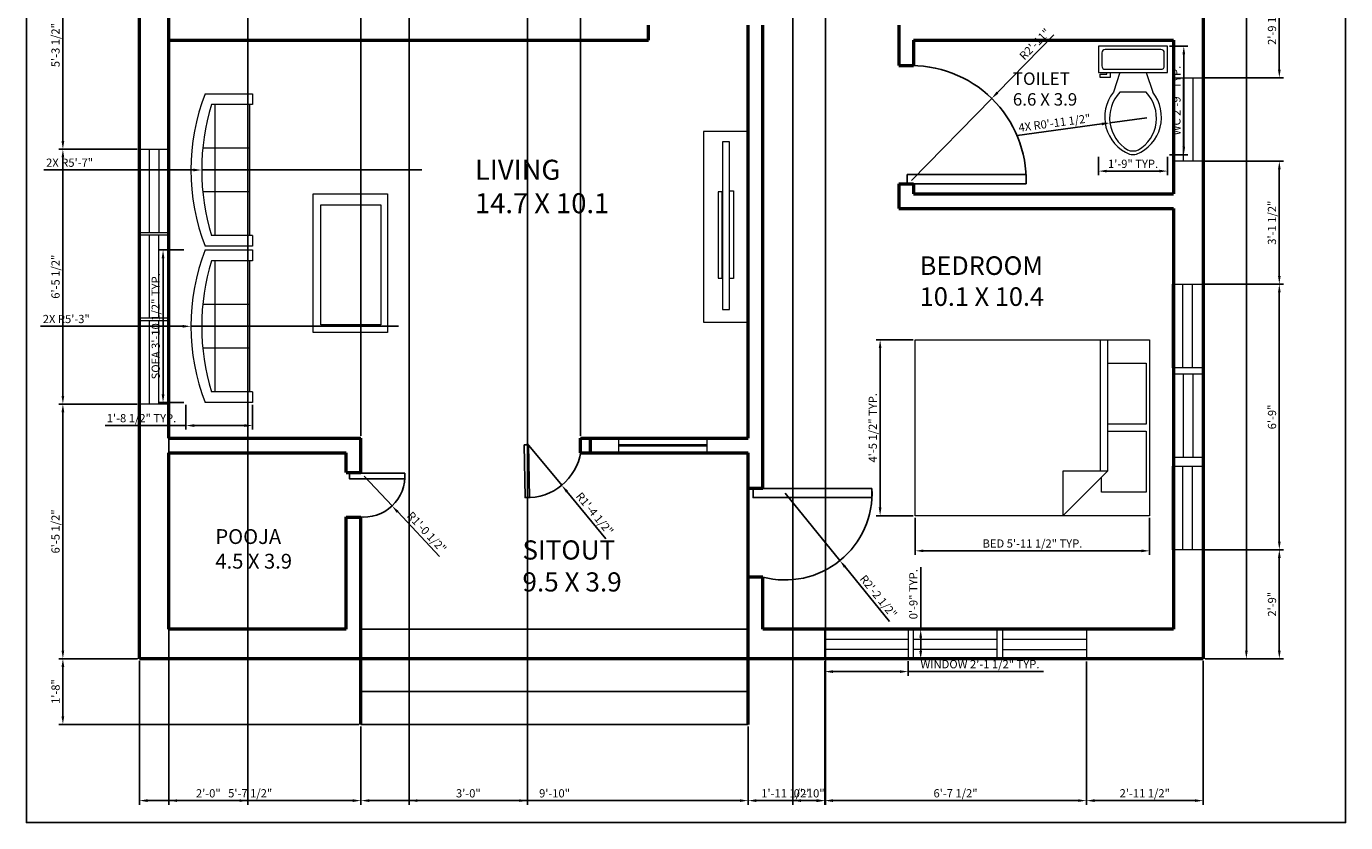
# Model space of a CAD drawing. Units: inches. Extents: x 231 to 633, y -1 to 510.
# Tile 1 of 3: x 231 to 633, y -1 to 242. Entities that reach past the tile are written whole.
import ezdxf

# ---------------------------------------------------------------- set-up
doc = ezdxf.new("R2010")
doc.units = ezdxf.units.IN
for name, color, linetype, lineweight in [('A-ANNO-DIMS', 2, 'Continuous', 18), ('A-ANNO-TTLB', 7, 'Continuous', 25), ('A-AREA-IDEN', 7, 'Continuous', 25), ('A-DOOR', 3, 'Continuous', 25), ('A-FLOR-FIXT', 9, 'Continuous', 18), ('A-FLOR-STRS', 7, 'Continuous', 25), ('A-FURN', 8, 'Continuous', 18), ('A-GLAZ', 4, 'Continuous', 18), ('A-WALL', 7, 'Continuous', 50)]:
    doc.layers.add(name, color=color, linetype=linetype, lineweight=lineweight)
doc.styles.get("Standard").update_dxf_attribs({"font": 'arial.ttf'})
doc.dimstyles.new('ISO-25', dxfattribs={"dimtxt": 2.5, "dimasz": 2.5, "dimexe": 1.25, "dimexo": 0.625, "dimtad": 1, "dimtxsty": 'Standard', "dimcen": 2.5, "dimadec": 0, "dimazin": 0, "dimtfac": 1, "dimtmove": 0, "dimatfit": 3, "dimfxl": 1, "dimarcsym": 0})

# ---------------------------------------------------------------- blocks, each defined once
blk = doc.blocks.new('Sofa - Roundback 7 ft.')
for p, q in [((-12.00002, -32.4421), (-12.00003, -6.5971)), ((11.99997, -32.4421), (11.99998, -6.5971)), ((-36.000027, -34), (-36.000027, -11.4696)), ((-35.999844, -13.3819), (35.9998, -13.3819)), ((35.99998, -34), (35.99998, -11.4696)), ((-36.000027, -32.4421), (35.99998, -32.4421))]:
    blk.add_line(p, q)
for points in [[(-36.000027, -34), (-42.000027, -34), (-42.000027, -8)], [(41.99998, -8), (41.99998, -34), (35.99998, -34)]]:
    blk.add_lwpolyline(points)
for centre, radius, start, end in [((0, -114.25), 114.25, 68.43141, 111.5686), ((-0.00001, -127.1968), 121.1968, 72.72033, 107.2797)]:
    blk.add_arc(centre, radius, start, end)
blk = doc.blocks.new('Toilet - top')
for p, q in [((9.5, -6), (9.5, -2)), ((-8, -8.5), (-8, -8)), ((-7, -8), (-7, -9.5)), ((-4, -8), (-6, -14)), ((4, -8), (6, -14)), ((-10, -8.5), (-8, -8.5)), ((-10, -9.5), (-10, -8.5)), ((-7, -9.5), (-10, -9.5)), ((4, -14), (-4, -14))]:
    blk.add_line(p, q)
blk.add_lwpolyline([(10.5, -8), (10.5, 0), (-10.5, 0), (-10.5, -8)], close=True)
for points in [[(-9.5, -2), (-9.5, -6)], [(8.5, -1), (-8.5, -1)], [(-8.5, -7), (8.5, -7)]]:
    blk.add_lwpolyline(points)
for centre, radius, start, end in [((-8.62, -1.88), 0.884, 81.8699, 188.1301), ((8.62, -1.88), 0.884, 351.8699, 98.1301), ((-8.62, -6.12), 0.884, 171.8699, 278.1301), ((8.62, -6.12), 0.884, 261.8699, 8.1301), ((3.52, -21.58), 12.17, 141.4691, 247.9714), ((4.2, -21.82), 11.33, 136.3677, 238.9468), ((-3.52, -21.58), 12.17, 292.0284, 38.5307), ((-4.2, -21.82), 11.33, 301.053, 43.6321), ((0, -27.88), 4, 245.7318, 294.2682), ((0, -29), 4, 254.8605, 285.1395)]:
    blk.add_arc(centre, radius, start, end)
blk = doc.blocks.new('Bed - Queen')
for p, q in [((0, -80.00003), (0, 0)), ((0, 0), (59.99999, 0)), ((59.99999, 0), (59.99999, -80.00003)), ((7.99999, -1.2), (28.79998, -1.2)), ((7.99999, -14.4), (7.99999, -1.2)), ((28.79998, -1.2), (28.79998, -14.4)), ((31.19999, -1.2), (51.99999, -1.2)), ((31.19999, -14.4), (31.19999, -1.2)), ((51.99999, -1.2), (51.99999, -16.4)), ((0, -14.4), (44.8, -14.4)), ((44.8, -16.8), (0, -16.8)), ((59.99999, -29.6), (44.8, -14.4)), ((44.8, -14.4), (44.8, -29.6)), ((51.99999, -16.4), (46.79936, -16.4)), ((44.8, -29.6), (59.99999, -29.6)), ((59.99999, -80.00003), (0, -80.00003))]:
    blk.add_line(p, q)
blk = doc.blocks.new('*D9')
at = {"layer": 'A-ANNO-DIMS', "color": 0, "lineweight": -2, "transparency": 16777216}
for p, q in [((589.91, 469.03), (603.7, 469.03)), ((602.45, 466.53), (602.45, 51.53)), ((589.91, 49.03), (603.7, 49.03))]:
    blk.add_line(p, q, dxfattribs=at)
at = {"layer": 'A-ANNO-DIMS', "color": 0, "transparency": 16777216}
for points in [[(602.04, 466.53), (602.87, 466.53), (602.45, 469.03)], [(602.04, 51.53), (602.87, 51.53), (602.45, 49.03)]]:
    blk.add_solid(points, dxfattribs=at)
at = {"layer": 'Defpoints', "color": 0, "transparency": 16777216}
for p in [(589.28, 469.03), (589.28, 49.03), (602.45, 49.03)]:
    blk.add_point(p, dxfattribs=at)
at = {"layer": 'A-ANNO-DIMS', "color": 0, "transparency": 16777216, "insert": (601.32, 259.03), "char_height": 1, "attachment_point": 5, "rotation": 90}
blk.add_mtext("35'", dxfattribs=at)
blk = doc.blocks.new('WIN-25_43x9')
for p, q in [((0, 0), (0, 9)), ((0, 9), (25.43, 9)), ((25.43, 9), (25.43, 0)), ((25.43, 6), (0, 6)), ((0, 3), (25.43, 3)), ((25.43, 0), (0, 0))]:
    blk.add_line(p, q)
blk = doc.blocks.new('*D12')
at = {"layer": 'A-ANNO-DIMS', "color": 0, "lineweight": -2, "transparency": 16777216}
for p, q in [((474.01, 48.31), (474.01, 43.87)), ((499.44, 48.31), (499.44, 43.87)), ((476.51, 45.12), (496.94, 45.12)), ((499.44, 45.12), (540.65, 45.12))]:
    blk.add_line(p, q, dxfattribs=at)
at = {"layer": 'A-ANNO-DIMS', "color": 0, "transparency": 16777216}
for points in [[(476.51, 45.53), (476.51, 44.7), (474.01, 45.12)], [(496.94, 45.53), (496.94, 44.7), (499.44, 45.12)]]:
    blk.add_solid(points, dxfattribs=at)
at = {"layer": 'Defpoints', "color": 0, "transparency": 16777216}
for p in [(474.01, 48.93), (499.44, 48.93), (499.44, 45.12)]:
    blk.add_point(p, dxfattribs=at)
at = {"layer": 'A-ANNO-DIMS', "color": 0, "transparency": 16777216, "insert": (521.3, 47.04), "char_height": 2.5, "attachment_point": 5}
blk.add_mtext('WINDOW 2\'-1 1/2" TYP.', dxfattribs=at)
blk = doc.blocks.new('*D13')
at = {"layer": 'A-ANNO-DIMS', "color": 0, "lineweight": -2, "transparency": 16777216}
for p, q in [((503.26, 57.93), (503.26, 76.92)), ((500.07, 57.93), (504.51, 57.93)), ((503.26, 51.43), (503.26, 55.43)), ((500.07, 48.93), (504.51, 48.93))]:
    blk.add_line(p, q, dxfattribs=at)
at = {"layer": 'A-ANNO-DIMS', "color": 0, "transparency": 16777216}
for points in [[(502.84, 55.43), (503.67, 55.43), (503.26, 57.93)], [(502.84, 51.43), (503.67, 51.43), (503.26, 48.93)]]:
    blk.add_solid(points, dxfattribs=at)
at = {"layer": 'Defpoints', "color": 0, "transparency": 16777216}
for p in [(499.44, 57.93), (503.26, 57.93), (499.44, 48.93)]:
    blk.add_point(p, dxfattribs=at)
at = {"layer": 'A-ANNO-DIMS', "color": 0, "transparency": 16777216, "insert": (501.35, 68.68), "char_height": 2.5, "attachment_point": 5, "rotation": 90}
blk.add_mtext('0\'-9" TYP.', dxfattribs=at)
blk = doc.blocks.new('*D14')
at = {"layer": 'A-ANNO-DIMS', "color": 0, "lineweight": -2, "transparency": 16777216}
for p, q in [((501.6, 91.97), (501.6, 80.64)), ((572.99, 91.97), (572.99, 80.64)), ((504.1, 81.89), (570.49, 81.89))]:
    blk.add_line(p, q, dxfattribs=at)
at = {"layer": 'A-ANNO-DIMS', "color": 0, "transparency": 16777216}
for points in [[(504.1, 82.3), (504.1, 81.47), (501.6, 81.89)], [(570.49, 82.3), (570.49, 81.47), (572.99, 81.89)]]:
    blk.add_solid(points, dxfattribs=at)
at = {"layer": 'Defpoints', "color": 0, "transparency": 16777216}
for p in [(501.6, 92.59), (572.99, 92.59), (572.99, 81.89)]:
    blk.add_point(p, dxfattribs=at)
at = {"layer": 'A-ANNO-DIMS', "color": 0, "transparency": 16777216, "insert": (537.3, 83.8), "char_height": 2.5, "attachment_point": 5}
blk.add_mtext('BED 5\'-11 1/2" TYP.', dxfattribs=at)
blk = doc.blocks.new('*D15')
at = {"layer": 'A-ANNO-DIMS', "color": 0, "lineweight": -2, "transparency": 16777216}
for p, q in [((500.98, 146.13), (489.65, 146.13)), ((490.9, 143.63), (490.9, 95.09)), ((500.98, 92.59), (489.65, 92.59))]:
    blk.add_line(p, q, dxfattribs=at)
at = {"layer": 'A-ANNO-DIMS', "color": 0, "transparency": 16777216}
for points in [[(490.48, 143.63), (491.31, 143.63), (490.9, 146.13)], [(490.48, 95.09), (491.31, 95.09), (490.9, 92.59)]]:
    blk.add_solid(points, dxfattribs=at)
at = {"layer": 'Defpoints', "color": 0, "transparency": 16777216}
for p in [(501.6, 146.13), (490.9, 92.59), (501.6, 92.59)]:
    blk.add_point(p, dxfattribs=at)
at = {"layer": 'A-ANNO-DIMS', "color": 0, "transparency": 16777216, "insert": (488.98, 119.36), "char_height": 2.5, "attachment_point": 5, "rotation": 90}
blk.add_mtext('4\'-5 1/2" TYP.', dxfattribs=at)
blk = doc.blocks.new('*D16')
at = {"layer": 'A-ANNO-DIMS', "color": 0, "lineweight": -2, "transparency": 16777216}
for p, q in [((579.07, 235.52), (584.65, 235.52)), ((583.4, 204.97), (583.4, 233.02)), ((579.07, 202.47), (584.65, 202.47))]:
    blk.add_line(p, q, dxfattribs=at)
at = {"layer": 'A-ANNO-DIMS', "color": 0, "transparency": 16777216}
for points in [[(582.98, 233.02), (583.82, 233.02), (583.4, 235.52)], [(582.98, 204.97), (583.82, 204.97), (583.4, 202.47)]]:
    blk.add_solid(points, dxfattribs=at)
at = {"layer": 'Defpoints', "color": 0, "transparency": 16777216}
for p in [(578.44, 235.52), (583.4, 235.52), (578.44, 202.47)]:
    blk.add_point(p, dxfattribs=at)
at = {"layer": 'A-ANNO-DIMS', "color": 0, "transparency": 16777216, "insert": (581.48, 218.99), "char_height": 2.5, "attachment_point": 5, "rotation": 90}
blk.add_mtext('WC 2\'-9" TYP.', dxfattribs=at)
blk = doc.blocks.new('*D17')
at = {"layer": 'A-ANNO-DIMS', "color": 0, "lineweight": -2, "transparency": 16777216}
for p, q in [((557.44, 201.85), (557.44, 196.26)), ((578.44, 201.85), (578.44, 196.26)), ((559.94, 197.51), (575.94, 197.51))]:
    blk.add_line(p, q, dxfattribs=at)
at = {"layer": 'A-ANNO-DIMS', "color": 0, "transparency": 16777216}
for points in [[(559.94, 197.93), (559.94, 197.1), (557.44, 197.51)], [(575.94, 197.93), (575.94, 197.1), (578.44, 197.51)]]:
    blk.add_solid(points, dxfattribs=at)
at = {"layer": 'Defpoints', "color": 0, "transparency": 16777216}
for p in [(557.44, 202.47), (578.44, 202.47), (578.44, 197.51)]:
    blk.add_point(p, dxfattribs=at)
at = {"layer": 'A-ANNO-DIMS', "color": 0, "transparency": 16777216, "insert": (567.94, 199.41), "char_height": 2.5, "attachment_point": 5}
blk.add_mtext('1\'-9" TYP.', dxfattribs=at)
blk = doc.blocks.new('*D18')
at = {"layer": 'A-ANNO-DIMS', "color": 0, "lineweight": -2, "transparency": 16777216}
for p, q in [((278.84, 173.5), (271.24, 173.5)), ((272.49, 129.51), (272.49, 171)), ((278.84, 127.01), (271.24, 127.01))]:
    blk.add_line(p, q, dxfattribs=at)
at = {"layer": 'A-ANNO-DIMS', "color": 0, "transparency": 16777216}
for points in [[(272.08, 171), (272.91, 171), (272.49, 173.5)], [(272.08, 129.51), (272.91, 129.51), (272.49, 127.01)]]:
    blk.add_solid(points, dxfattribs=at)
at = {"layer": 'Defpoints', "color": 0, "transparency": 16777216}
for p in [(272.49, 173.5), (279.47, 173.5), (279.47, 127.01)]:
    blk.add_point(p, dxfattribs=at)
at = {"layer": 'A-ANNO-DIMS', "color": 0, "transparency": 16777216, "insert": (270.58, 150.26), "char_height": 2.5, "attachment_point": 5, "rotation": 90}
blk.add_mtext('SOFA 3\'-10 1/2" TYP.', dxfattribs=at)
blk = doc.blocks.new('*D19')
at = {"layer": 'A-ANNO-DIMS', "color": 0, "lineweight": -2, "transparency": 16777216}
for p, q in [((279.47, 126.39), (279.47, 118.79)), ((299.76, 126.39), (299.76, 118.79)), ((279.47, 120.04), (254.89, 120.04)), ((297.26, 120.04), (281.97, 120.04))]:
    blk.add_line(p, q, dxfattribs=at)
at = {"layer": 'A-ANNO-DIMS', "color": 0, "transparency": 16777216}
for points in [[(281.97, 120.46), (281.97, 119.62), (279.47, 120.04)], [(297.26, 120.46), (297.26, 119.62), (299.76, 120.04)]]:
    blk.add_solid(points, dxfattribs=at)
at = {"layer": 'Defpoints', "color": 0, "transparency": 16777216}
for p in [(279.47, 127.01), (299.76, 127.01), (279.47, 120.04)]:
    blk.add_point(p, dxfattribs=at)
at = {"layer": 'A-ANNO-DIMS', "color": 0, "transparency": 16777216, "insert": (265.93, 121.96), "char_height": 2.5, "attachment_point": 5}
blk.add_mtext('1\'-8 1/2" TYP.', dxfattribs=at)
blk = doc.blocks.new('*D30')
at = {"layer": 'A-ANNO-DIMS', "color": 0, "lineweight": -2, "transparency": 16777216}
for p, q in [((264.66, 49.03), (240.73, 49.03)), ((241.98, 31.53), (241.98, 46.53)), ((332.16, 29.03), (240.73, 29.03))]:
    blk.add_line(p, q, dxfattribs=at)
at = {"layer": 'A-ANNO-DIMS', "color": 0, "transparency": 16777216}
for points in [[(241.56, 46.53), (242.4, 46.53), (241.98, 49.03)], [(241.56, 31.53), (242.4, 31.53), (241.98, 29.03)]]:
    blk.add_solid(points, dxfattribs=at)
at = {"layer": 'Defpoints', "color": 0, "transparency": 16777216}
for p in [(241.98, 49.03), (265.28, 49.03), (332.78, 29.03)]:
    blk.add_point(p, dxfattribs=at)
at = {"layer": 'A-ANNO-DIMS', "color": 0, "transparency": 16777216, "insert": (240.08, 39.03), "char_height": 2.5, "attachment_point": 5, "rotation": 90}
blk.add_mtext('1\'-8"', dxfattribs=at)
blk = doc.blocks.new('*D31')
at = {"layer": 'A-ANNO-DIMS', "color": 0, "lineweight": -2, "transparency": 16777216}
for p, q in [((265.28, 48.41), (265.28, 4.58)), ((332.78, 28.41), (332.78, 4.58)), ((267.78, 5.83), (330.28, 5.83))]:
    blk.add_line(p, q, dxfattribs=at)
at = {"layer": 'A-ANNO-DIMS', "color": 0, "transparency": 16777216}
for points in [[(267.78, 6.25), (267.78, 5.42), (265.28, 5.83)], [(330.28, 6.25), (330.28, 5.42), (332.78, 5.83)]]:
    blk.add_solid(points, dxfattribs=at)
at = {"layer": 'Defpoints', "color": 0, "transparency": 16777216}
for p in [(265.28, 49.03), (332.78, 29.03), (332.78, 5.83)]:
    blk.add_point(p, dxfattribs=at)
at = {"layer": 'A-ANNO-DIMS', "color": 0, "transparency": 16777216, "insert": (299.03, 7.75), "char_height": 2.5, "attachment_point": 5}
blk.add_mtext('5\'-7 1/2"', dxfattribs=at)
blk = doc.blocks.new('*D32')
at = {"layer": 'A-ANNO-DIMS', "color": 0, "lineweight": -2, "transparency": 16777216}
for p, q in [((332.78, 28.41), (332.78, 4.58)), ((450.68, 28.41), (450.68, 4.58)), ((335.28, 5.83), (448.18, 5.83))]:
    blk.add_line(p, q, dxfattribs=at)
at = {"layer": 'A-ANNO-DIMS', "color": 0, "transparency": 16777216}
for points in [[(335.28, 6.25), (335.28, 5.42), (332.78, 5.83)], [(448.18, 6.25), (448.18, 5.42), (450.68, 5.83)]]:
    blk.add_solid(points, dxfattribs=at)
at = {"layer": 'Defpoints', "color": 0, "transparency": 16777216}
for p in [(332.78, 29.03), (450.68, 29.03), (450.68, 5.83)]:
    blk.add_point(p, dxfattribs=at)
at = {"layer": 'A-ANNO-DIMS', "color": 0, "transparency": 16777216, "insert": (391.73, 7.73), "char_height": 2.5, "attachment_point": 5}
blk.add_mtext('9\'-10"', dxfattribs=at)
blk = doc.blocks.new('*D35')
at = {"layer": 'A-ANNO-DIMS', "color": 0, "lineweight": -2, "transparency": 16777216}
for p, q in [((464.28, 330.11), (464.28, 4.58)), ((474.28, 330.11), (474.28, 4.58)), ((466.78, 5.83), (471.78, 5.83))]:
    blk.add_line(p, q, dxfattribs=at)
at = {"layer": 'A-ANNO-DIMS', "color": 0, "transparency": 16777216}
for points in [[(466.78, 6.25), (466.78, 5.42), (464.28, 5.83)], [(471.78, 6.25), (471.78, 5.42), (474.28, 5.83)]]:
    blk.add_solid(points, dxfattribs=at)
at = {"layer": 'Defpoints', "color": 0, "transparency": 16777216}
for p in [(464.28, 330.73), (474.28, 330.73), (474.28, 5.83)]:
    blk.add_point(p, dxfattribs=at)
at = {"layer": 'A-ANNO-DIMS', "color": 0, "transparency": 16777216, "insert": (469.28, 7.73), "char_height": 2.5, "attachment_point": 5}
blk.add_mtext('0\'-10"', dxfattribs=at)
blk = doc.blocks.new('*D41')
at = {"layer": 'A-ANNO-DIMS', "color": 0, "lineweight": -2, "transparency": 16777216}
for p, q in [((274.28, 349.01), (274.28, 4.58)), ((298.28, 349.01), (298.28, 4.58)), ((276.78, 5.83), (295.78, 5.83))]:
    blk.add_line(p, q, dxfattribs=at)
at = {"layer": 'A-ANNO-DIMS', "color": 0, "transparency": 16777216}
for points in [[(276.78, 6.25), (276.78, 5.42), (274.28, 5.83)], [(295.78, 6.25), (295.78, 5.42), (298.28, 5.83)]]:
    blk.add_solid(points, dxfattribs=at)
at = {"layer": 'Defpoints', "color": 0, "transparency": 16777216}
for p in [(274.28, 349.63), (298.28, 349.63), (298.28, 5.83)]:
    blk.add_point(p, dxfattribs=at)
at = {"layer": 'A-ANNO-DIMS', "color": 0, "transparency": 16777216, "insert": (286.28, 7.73), "char_height": 2.5, "attachment_point": 5}
blk.add_mtext('2\'-0"', dxfattribs=at)
blk = doc.blocks.new('*D42')
at = {"layer": 'A-ANNO-DIMS', "color": 0, "lineweight": -2, "transparency": 16777216}
for p, q in [((347.48, 344.51), (347.48, 4.58)), ((383.48, 330.11), (383.48, 4.58)), ((349.98, 5.83), (380.98, 5.83))]:
    blk.add_line(p, q, dxfattribs=at)
at = {"layer": 'A-ANNO-DIMS', "color": 0, "transparency": 16777216}
for points in [[(349.98, 6.25), (349.98, 5.42), (347.48, 5.83)], [(380.98, 6.25), (380.98, 5.42), (383.48, 5.83)]]:
    blk.add_solid(points, dxfattribs=at)
at = {"layer": 'Defpoints', "color": 0, "transparency": 16777216}
for p in [(347.48, 345.13), (383.48, 330.73), (383.48, 5.83)]:
    blk.add_point(p, dxfattribs=at)
at = {"layer": 'A-ANNO-DIMS', "color": 0, "transparency": 16777216, "insert": (365.48, 7.73), "char_height": 2.5, "attachment_point": 5}
blk.add_mtext('3\'-0"', dxfattribs=at)
blk = doc.blocks.new('*D43')
at = {"layer": 'A-ANNO-DIMS', "color": 0, "lineweight": -2, "transparency": 16777216}
for p, q in [((264.62, 126.57), (240.73, 126.57)), ((241.98, 51.53), (241.98, 124.07)), ((264.66, 49.03), (240.73, 49.03))]:
    blk.add_line(p, q, dxfattribs=at)
at = {"layer": 'A-ANNO-DIMS', "color": 0, "transparency": 16777216}
for points in [[(241.56, 124.07), (242.4, 124.07), (241.98, 126.57)], [(241.56, 51.53), (242.4, 51.53), (241.98, 49.03)]]:
    blk.add_solid(points, dxfattribs=at)
at = {"layer": 'Defpoints', "color": 0, "transparency": 16777216}
for p in [(241.98, 126.57), (265.25, 126.57), (265.28, 49.03)]:
    blk.add_point(p, dxfattribs=at)
at = {"layer": 'A-ANNO-DIMS', "color": 0, "transparency": 16777216, "insert": (240.06, 87.8), "char_height": 2.5, "attachment_point": 5, "rotation": 90}
blk.add_mtext('6\'-5 1/2"', dxfattribs=at)
blk = doc.blocks.new('*D44')
at = {"layer": 'A-ANNO-DIMS', "color": 0, "lineweight": -2, "transparency": 16777216}
for p, q in [((264.65, 204.16), (240.73, 204.16)), ((241.98, 129.07), (241.98, 201.66)), ((264.62, 126.57), (240.73, 126.57))]:
    blk.add_line(p, q, dxfattribs=at)
at = {"layer": 'A-ANNO-DIMS', "color": 0, "transparency": 16777216}
for points in [[(241.56, 201.66), (242.4, 201.66), (241.98, 204.16)], [(241.56, 129.07), (242.4, 129.07), (241.98, 126.57)]]:
    blk.add_solid(points, dxfattribs=at)
at = {"layer": 'Defpoints', "color": 0, "transparency": 16777216}
for p in [(241.98, 204.16), (265.27, 204.16), (265.25, 126.57)]:
    blk.add_point(p, dxfattribs=at)
at = {"layer": 'A-ANNO-DIMS', "color": 0, "transparency": 16777216, "insert": (240.06, 165.36), "char_height": 2.5, "attachment_point": 5, "rotation": 90}
blk.add_mtext('6\'-5 1/2"', dxfattribs=at)
blk = doc.blocks.new('*D45')
at = {"layer": 'A-ANNO-DIMS', "color": 0, "lineweight": -2, "transparency": 16777216}
for p, q in [((264.59, 267.58), (240.73, 267.58)), ((241.98, 206.66), (241.98, 265.08)), ((264.65, 204.16), (240.73, 204.16))]:
    blk.add_line(p, q, dxfattribs=at)
at = {"layer": 'A-ANNO-DIMS', "color": 0, "transparency": 16777216}
for points in [[(241.56, 265.08), (242.4, 265.08), (241.98, 267.58)], [(241.56, 206.66), (242.4, 206.66), (241.98, 204.16)]]:
    blk.add_solid(points, dxfattribs=at)
at = {"layer": 'Defpoints', "color": 0, "transparency": 16777216}
for p in [(241.98, 267.58), (265.22, 267.58), (265.27, 204.16)]:
    blk.add_point(p, dxfattribs=at)
at = {"layer": 'A-ANNO-DIMS', "color": 0, "transparency": 16777216, "insert": (240.06, 235.87), "char_height": 2.5, "attachment_point": 5, "rotation": 90}
blk.add_mtext('5\'-3 1/2"', dxfattribs=at)
blk = doc.blocks.new('*D50')
at = {"layer": 'A-ANNO-DIMS', "color": 0, "lineweight": -2, "transparency": 16777216}
for p, q in [((589.63, 82.23), (613.74, 82.23)), ((612.49, 51.53), (612.49, 79.73)), ((589.91, 49.03), (613.74, 49.03))]:
    blk.add_line(p, q, dxfattribs=at)
at = {"layer": 'A-ANNO-DIMS', "color": 0, "transparency": 16777216}
for points in [[(612.08, 79.73), (612.91, 79.73), (612.49, 82.23)], [(612.08, 51.53), (612.91, 51.53), (612.49, 49.03)]]:
    blk.add_solid(points, dxfattribs=at)
at = {"layer": 'Defpoints', "color": 0, "transparency": 16777216}
for p in [(589, 82.23), (612.49, 82.23), (589.28, 49.03)]:
    blk.add_point(p, dxfattribs=at)
at = {"layer": 'A-ANNO-DIMS', "color": 0, "transparency": 16777216, "insert": (610.59, 65.63), "char_height": 2.5, "attachment_point": 5, "rotation": 90}
blk.add_mtext('2\'-9"', dxfattribs=at)
blk = doc.blocks.new('*D51')
at = {"layer": 'A-ANNO-DIMS', "color": 0, "lineweight": -2, "transparency": 16777216}
for p, q in [((589.63, 163.09), (613.74, 163.09)), ((612.49, 84.73), (612.49, 160.59)), ((589.63, 82.23), (613.74, 82.23))]:
    blk.add_line(p, q, dxfattribs=at)
at = {"layer": 'A-ANNO-DIMS', "color": 0, "transparency": 16777216}
for points in [[(612.08, 160.59), (612.91, 160.59), (612.49, 163.09)], [(612.08, 84.73), (612.91, 84.73), (612.49, 82.23)]]:
    blk.add_solid(points, dxfattribs=at)
at = {"layer": 'Defpoints', "color": 0, "transparency": 16777216}
for p in [(589, 163.09), (612.49, 163.09), (589, 82.23)]:
    blk.add_point(p, dxfattribs=at)
at = {"layer": 'A-ANNO-DIMS', "color": 0, "transparency": 16777216, "insert": (610.59, 122.66), "char_height": 2.5, "attachment_point": 5, "rotation": 90}
blk.add_mtext('6\'-9"', dxfattribs=at)
blk = doc.blocks.new('*D52')
at = {"layer": 'A-ANNO-DIMS', "color": 0, "lineweight": -2, "transparency": 16777216}
for p, q in [((589.84, 200.51), (613.74, 200.51)), ((612.49, 165.59), (612.49, 198.01)), ((589.63, 163.09), (613.74, 163.09))]:
    blk.add_line(p, q, dxfattribs=at)
at = {"layer": 'A-ANNO-DIMS', "color": 0, "transparency": 16777216}
for points in [[(612.08, 198.01), (612.91, 198.01), (612.49, 200.51)], [(612.08, 165.59), (612.91, 165.59), (612.49, 163.09)]]:
    blk.add_solid(points, dxfattribs=at)
at = {"layer": 'Defpoints', "color": 0, "transparency": 16777216}
for p in [(589.22, 200.51), (612.49, 200.51), (589, 163.09)]:
    blk.add_point(p, dxfattribs=at)
at = {"layer": 'A-ANNO-DIMS', "color": 0, "transparency": 16777216, "insert": (610.57, 181.8), "char_height": 2.5, "attachment_point": 5, "rotation": 90}
blk.add_mtext('3\'-1 1/2"', dxfattribs=at)
blk = doc.blocks.new('*D53')
at = {"layer": 'A-ANNO-DIMS', "color": 0, "lineweight": -2, "transparency": 16777216}
for p, q in [((589.78, 259.34), (613.74, 259.34)), ((612.49, 228.44), (612.49, 256.84)), ((589.84, 225.94), (613.74, 225.94))]:
    blk.add_line(p, q, dxfattribs=at)
at = {"layer": 'A-ANNO-DIMS', "color": 0, "transparency": 16777216}
for points in [[(612.08, 256.84), (612.91, 256.84), (612.49, 259.34)], [(612.08, 228.44), (612.91, 228.44), (612.49, 225.94)]]:
    blk.add_solid(points, dxfattribs=at)
at = {"layer": 'Defpoints', "color": 0, "transparency": 16777216}
for p in [(589.15, 259.34), (612.49, 259.34), (589.22, 225.94)]:
    blk.add_point(p, dxfattribs=at)
at = {"layer": 'A-ANNO-DIMS', "color": 0, "transparency": 16777216, "insert": (610.58, 242.64), "char_height": 2.5, "attachment_point": 5, "rotation": 90}
blk.add_mtext('2\'-9 1/2"', dxfattribs=at)
blk = doc.blocks.new('*D61')
at = {"layer": 'A-ANNO-DIMS', "color": 0, "lineweight": -2, "transparency": 16777216}
for p, q in [((474.01, 48.31), (474.01, 4.58)), ((450.68, 28.41), (450.68, 4.58)), ((453.18, 5.83), (471.51, 5.83))]:
    blk.add_line(p, q, dxfattribs=at)
at = {"layer": 'A-ANNO-DIMS', "color": 0, "transparency": 16777216}
for points in [[(453.18, 6.25), (453.18, 5.42), (450.68, 5.83)], [(471.51, 6.25), (471.51, 5.42), (474.01, 5.83)]]:
    blk.add_solid(points, dxfattribs=at)
at = {"layer": 'Defpoints', "color": 0, "transparency": 16777216}
for p in [(474.01, 48.93), (450.68, 29.03), (474.01, 5.83)]:
    blk.add_point(p, dxfattribs=at)
at = {"layer": 'A-ANNO-DIMS', "color": 0, "transparency": 16777216, "insert": (462.35, 7.75), "char_height": 2.5, "attachment_point": 5}
blk.add_mtext('1\'-11 1/2"', dxfattribs=at)
blk = doc.blocks.new('*D62')
at = {"layer": 'A-ANNO-DIMS', "color": 0, "lineweight": -2, "transparency": 16777216}
for p, q in [((553.73, 48.23), (553.73, 4.58)), ((589.28, 48.41), (589.28, 4.58)), ((556.23, 5.83), (586.78, 5.83))]:
    blk.add_line(p, q, dxfattribs=at)
at = {"layer": 'A-ANNO-DIMS', "color": 0, "transparency": 16777216}
for points in [[(556.23, 6.25), (556.23, 5.42), (553.73, 5.83)], [(586.78, 6.25), (586.78, 5.42), (589.28, 5.83)]]:
    blk.add_solid(points, dxfattribs=at)
at = {"layer": 'Defpoints', "color": 0, "transparency": 16777216}
for p in [(553.73, 48.85), (589.28, 49.03), (589.28, 5.83)]:
    blk.add_point(p, dxfattribs=at)
at = {"layer": 'A-ANNO-DIMS', "color": 0, "transparency": 16777216, "insert": (571.5, 7.75), "char_height": 2.5, "attachment_point": 5}
blk.add_mtext('2\'-11 1/2"', dxfattribs=at)
blk = doc.blocks.new('*D63')
at = {"layer": 'A-ANNO-DIMS', "color": 0, "lineweight": -2, "transparency": 16777216}
for p, q in [((474.01, 48.31), (474.01, 4.58)), ((553.73, 48.23), (553.73, 4.58)), ((476.51, 5.83), (551.23, 5.83))]:
    blk.add_line(p, q, dxfattribs=at)
at = {"layer": 'A-ANNO-DIMS', "color": 0, "transparency": 16777216}
for points in [[(476.51, 6.25), (476.51, 5.42), (474.01, 5.83)], [(551.23, 6.25), (551.23, 5.42), (553.73, 5.83)]]:
    blk.add_solid(points, dxfattribs=at)
at = {"layer": 'Defpoints', "color": 0, "transparency": 16777216}
for p in [(474.01, 48.93), (553.73, 48.85), (553.73, 5.83)]:
    blk.add_point(p, dxfattribs=at)
at = {"layer": 'A-ANNO-DIMS', "color": 0, "transparency": 16777216, "insert": (513.87, 7.75), "char_height": 2.5, "attachment_point": 5}
blk.add_mtext('6\'-7 1/2"', dxfattribs=at)
blk = doc.blocks.new('*D65')
at = {"layer": 'A-ANNO-DIMS', "color": 0, "lineweight": -2, "transparency": 16777216}
for p, q in [((332.78, 116.86), (332.78, 493.62)), ((335.28, 492.37), (397.18, 492.37)), ((399.68, 116.86), (399.68, 493.62))]:
    blk.add_line(p, q, dxfattribs=at)
at = {"layer": 'A-ANNO-DIMS', "color": 0, "transparency": 16777216}
for points in [[(335.28, 492.78), (335.28, 491.95), (332.78, 492.37)], [(397.18, 492.78), (397.18, 491.95), (399.68, 492.37)]]:
    blk.add_solid(points, dxfattribs=at)
at = {"layer": 'Defpoints', "color": 0, "transparency": 16777216}
for p in [(399.68, 492.37), (332.78, 116.23), (399.68, 116.23)]:
    blk.add_point(p, dxfattribs=at)
at = {"layer": 'A-ANNO-DIMS', "color": 0, "transparency": 16777216, "insert": (366.23, 494.26), "char_height": 2.5, "attachment_point": 5}
blk.add_mtext('5\'-7"', dxfattribs=at)
blk = doc.blocks.new('*D66')
at = {"layer": 'A-ANNO-DIMS', "color": 0, "lineweight": -2, "transparency": 16777216}
for p, q in [((543.86, 238.98), (526.64, 221.42)), ((500.42, 194.67), (524.89, 219.64))]:
    blk.add_line(p, q, dxfattribs=at)
at = {"layer": 'A-ANNO-DIMS', "color": 0, "transparency": 16777216}
blk.add_solid([(526.35, 221.71), (526.94, 221.13), (524.89, 219.64)], dxfattribs=at)
at = {"layer": 'Defpoints', "color": 0, "transparency": 16777216}
for p in [(524.89, 219.64), (500.42, 194.67)]:
    blk.add_point(p, dxfattribs=at)
at = {"layer": 'A-ANNO-DIMS', "color": 0, "transparency": 16777216, "insert": (538.24, 235.93), "char_height": 2.5, "attachment_point": 5, "rotation": 45.5699}
blk.add_mtext('R2\'-11"', dxfattribs=at)
blk = doc.blocks.new('*D69')
at = {"layer": 'A-ANNO-DIMS', "color": 0, "lineweight": -2, "transparency": 16777216}
for p, q in [((461.99, 99.49), (478.65, 78.93)), ((493.72, 60.33), (480.22, 76.99))]:
    blk.add_line(p, q, dxfattribs=at)
at = {"layer": 'A-ANNO-DIMS', "color": 0, "transparency": 16777216}
blk.add_solid([(480.55, 77.25), (479.9, 76.72), (478.65, 78.93)], dxfattribs=at)
at = {"layer": 'Defpoints', "color": 0, "transparency": 16777216}
for p in [(461.99, 99.49), (478.65, 78.93)]:
    blk.add_point(p, dxfattribs=at)
at = {"layer": 'A-ANNO-DIMS', "color": 0, "transparency": 16777216, "insert": (490.14, 67.8), "char_height": 2.5, "attachment_point": 5, "rotation": 309.0212}
blk.add_mtext('R2\'-2 1/2"', dxfattribs=at)
blk = doc.blocks.new('*D70')
at = {"layer": 'A-ANNO-DIMS', "color": 0, "lineweight": -2, "transparency": 16777216}
for p, q in [((383.44, 114.59), (393.92, 101.86)), ((407.34, 85.56), (395.51, 99.93))]:
    blk.add_line(p, q, dxfattribs=at)
at = {"layer": 'A-ANNO-DIMS', "color": 0, "transparency": 16777216}
blk.add_solid([(395.83, 100.19), (395.19, 99.66), (393.92, 101.86)], dxfattribs=at)
at = {"layer": 'Defpoints', "color": 0, "transparency": 16777216}
for p in [(383.44, 114.59), (393.92, 101.86)]:
    blk.add_point(p, dxfattribs=at)
at = {"layer": 'A-ANNO-DIMS', "color": 0, "transparency": 16777216, "insert": (403.7, 93), "char_height": 2.5, "attachment_point": 5, "rotation": 309.4659}
blk.add_mtext('R1\'-4 1/2"', dxfattribs=at)
blk = doc.blocks.new('*D71')
at = {"layer": 'A-ANNO-DIMS', "color": 0, "lineweight": -2, "transparency": 16777216}
for p, q in [((333.74, 104.6), (342.24, 95.55)), ((356.7, 80.17), (343.96, 93.73))]:
    blk.add_line(p, q, dxfattribs=at)
at = {"layer": 'A-ANNO-DIMS', "color": 0, "transparency": 16777216}
blk.add_solid([(344.26, 94.02), (343.65, 93.45), (342.24, 95.55)], dxfattribs=at)
at = {"layer": 'Defpoints', "color": 0, "transparency": 16777216}
for p in [(333.74, 104.6), (342.24, 95.55)]:
    blk.add_point(p, dxfattribs=at)
at = {"layer": 'A-ANNO-DIMS', "color": 0, "transparency": 16777216, "insert": (352.58, 87.35), "char_height": 2.5, "attachment_point": 5, "rotation": 313.2146}
blk.add_mtext('R1\'-0 1/2"', dxfattribs=at)
blk = doc.blocks.new('*D72')
at = {"layer": 'A-ANNO-DIMS', "color": 0, "lineweight": -2, "transparency": 16777216}
for p, q in [((236.17, 197.85), (281.76, 197.85)), ((351.33, 197.85), (284.26, 197.85))]:
    blk.add_line(p, q, dxfattribs=at)
at = {"layer": 'A-ANNO-DIMS', "color": 0, "transparency": 16777216}
blk.add_solid([(281.76, 198.27), (281.76, 197.44), (284.26, 197.85)], dxfattribs=at)
at = {"layer": 'Defpoints', "color": 0, "transparency": 16777216}
for p in [(284.26, 197.85), (351.33, 197.85)]:
    blk.add_point(p, dxfattribs=at)
at = {"layer": 'A-ANNO-DIMS', "color": 0, "transparency": 16777216, "insert": (244.02, 199.75), "char_height": 2.5, "attachment_point": 5, "rotation": 0.0001}
blk.add_mtext('2X R5\'-7"', dxfattribs=at)
blk = doc.blocks.new('*D73')
at = {"layer": 'A-ANNO-DIMS', "color": 0, "lineweight": -2, "transparency": 16777216}
for p, q in [((235.16, 150.26), (278.44, 150.26)), ((344.17, 150.26), (280.94, 150.26))]:
    blk.add_line(p, q, dxfattribs=at)
at = {"layer": 'A-ANNO-DIMS', "color": 0, "transparency": 16777216}
blk.add_solid([(278.44, 150.67), (278.44, 149.84), (280.94, 150.26)], dxfattribs=at)
at = {"layer": 'Defpoints', "color": 0, "transparency": 16777216}
for p in [(280.94, 150.26), (344.17, 150.26)]:
    blk.add_point(p, dxfattribs=at)
at = {"layer": 'A-ANNO-DIMS', "color": 0, "transparency": 16777216, "insert": (243.01, 152.16), "char_height": 2.5, "attachment_point": 5}
blk.add_mtext('2X R5\'-3"', dxfattribs=at)
blk = doc.blocks.new('*D75')
at = {"layer": 'A-ANNO-DIMS', "color": 0, "lineweight": -2, "transparency": 16777216}
for p, q in [((572.14, 213.7), (560.91, 212.19)), ((532.64, 208.39), (558.44, 211.86))]:
    blk.add_line(p, q, dxfattribs=at)
at = {"layer": 'A-ANNO-DIMS', "color": 0, "transparency": 16777216}
blk.add_solid([(558.38, 212.27), (558.49, 211.44), (560.91, 212.19)], dxfattribs=at)
at = {"layer": 'Defpoints', "color": 0, "transparency": 16777216}
for p in [(572.14, 213.7), (560.91, 212.19)]:
    blk.add_point(p, dxfattribs=at)
at = {"layer": 'A-ANNO-DIMS', "color": 0, "transparency": 16777216, "insert": (544.04, 211.86), "char_height": 2.5, "attachment_point": 5, "rotation": 7.6557}
blk.add_mtext('4X R0\'-11 1/2"', dxfattribs=at)

msp = doc.modelspace()

# ---------------------------------------------------------------- linework, layer by layer
at = {"layer": 'A-ANNO-TTLB'}
msp.add_lwpolyline([(230.86, 510.42), (632.68, 510.42), (632.68, -0.86), (230.86, -0.86)], close=True, dxfattribs=at)
at = {"layer": 'A-DOOR'}
for points in [[(535.37, 196.43), (535.37, 193.68), (499.17, 193.68), (499.17, 196.43)], [(384.11, 98.11), (382.76, 98.11), (382.51, 114.14), (383.85, 114.14)], [(346.13, 105.52), (346.13, 103.85), (329.27, 103.85), (329.27, 105.52)], [(488.42, 100.86), (488.42, 98.12), (452.21, 98.12), (452.21, 100.86)]]:
    msp.add_lwpolyline(points, close=True, dxfattribs=at)
for centre, radius, start, end in [((500.42, 194.67), 34.96, 358.3635, 92.7769), ((383.44, 114.59), 16.49, 267.6488, 351.2829), ((333.74, 104.6), 12.42, 262.1598, 4.268), ((461.99, 99.49), 26.47, 255.0643, 2.9785)]:
    msp.add_arc(centre, radius, start, end, dxfattribs=at)
at = {"layer": 'A-FLOR-STRS'}
for p, q in [((450.68, 58.03), (332.78, 58.03)), ((450.68, 39.03), (332.78, 39.03)), ((450.68, 29.03), (332.78, 29.03))]:
    msp.add_line(p, q, dxfattribs=at)
at = {"layer": 'A-FURN'}
for points in [[(450.56, 209.54), (437.09, 209.54), (437.09, 151.48), (450.56, 151.48)], [(445.02, 206.42), (442.84, 206.42), (442.84, 155.37), (445.02, 155.37)], [(318.24, 190.64), (340.82, 190.64), (340.82, 148.34), (318.24, 148.34)], [(442.83, 191.24), (441.57, 191.24), (441.57, 164.88), (442.83, 164.88)], [(445.04, 191.54), (446.27, 191.54), (446.27, 164.83), (445.04, 164.83)], [(320.54, 187.27), (338.83, 187.27), (338.83, 150.71), (320.54, 150.71)]]:
    msp.add_lwpolyline(points, close=True, dxfattribs=at)
at = {"layer": 'A-GLAZ'}
for p, q in [((411.28, 111.74), (411.28, 116.24)), ((411.28, 116.24), (438.14, 116.24)), ((411.28, 114.24), (438.14, 114.24)), ((438.14, 113.74), (411.28, 113.74)), ((438.14, 116.24), (438.14, 111.74)), ((438.14, 111.74), (411.28, 111.74))]:
    msp.add_line(p, q, dxfattribs=at)
at = {"layer": 'A-WALL'}
for p, q in [((265.28, 49.03), (265.28, 469.03)), ((589.28, 469.03), (589.28, 49.03)), ((274.28, 116.23), (274.28, 345.13)), ((420.38, 237.43), (420.38, 241.93)), ((450.68, 116.23), (450.68, 241.93)), ((455.18, 100.93), (455.18, 241.93)), ((496.58, 241.93), (496.58, 229.63)), ((274.28, 237.43), (420.38, 237.43)), ((501.08, 237.43), (580.28, 237.43)), ((501.08, 237.43), (501.08, 229.63)), ((580.28, 237.43), (580.28, 190.63)), ((496.58, 229.63), (501.08, 229.63)), ((496.58, 193.63), (501.08, 193.63)), ((496.58, 193.63), (496.58, 186.13)), ((501.08, 193.63), (501.08, 190.63)), ((501.08, 190.63), (580.28, 190.63)), ((496.58, 186.13), (580.28, 186.13)), ((580.28, 186.13), (580.28, 58.03)), ((274.28, 116.23), (332.78, 116.23)), ((332.78, 105.73), (332.78, 116.23)), ((399.68, 116.23), (450.68, 116.23)), ((399.68, 111.73), (399.68, 116.23)), ((402.68, 111.73), (402.68, 116.23)), ((274.28, 58.03), (274.28, 111.73)), ((274.28, 111.73), (328.28, 111.73)), ((328.28, 105.73), (328.28, 111.73)), ((399.68, 111.73), (450.68, 111.73)), ((450.68, 100.93), (450.68, 111.73)), ((328.28, 105.73), (332.78, 105.73)), ((450.68, 29.03), (450.68, 100.93)), ((450.68, 100.93), (455.18, 100.93)), ((328.28, 58.03), (328.28, 92.26)), ((328.28, 92.17), (332.78, 92.17)), ((332.78, 29.03), (332.78, 92.22)), ((450.68, 73.93), (455.18, 73.93)), ((455.18, 58.03), (455.18, 73.93)), ((328.28, 58.03), (274.28, 58.03)), ((580.28, 58.03), (455.18, 58.03)), ((589.28, 49.03), (265.28, 49.03))]:
    msp.add_line(p, q, dxfattribs=at)

# ---------------------------------------------------------------- block references
at = {"layer": 'A-FLOR-FIXT'}
msp.add_blockref('Toilet - top', (567.94, 235.52), dxfattribs=at)
at = {"layer": 'A-FURN'}
for name, p, xscale, yscale, zscale, rotation in [('Sofa - Roundback 7 ft.', (280.94, 197.85), 0.5533813357364022, 0.5533813357364022, 0.5533813357364022, 90), ('Sofa - Roundback 7 ft.', (280.94, 150.26), 0.5533813357364022, 0.5533813357364022, 0.5533813357364022, 90), ('Bed - Queen', (572.99, 146.13), 0.8923370876530633, 0.8923370876530633, 0.8923370876530633, 270)]:
    msp.add_blockref(name, p, dxfattribs=dict(at, xscale=xscale, yscale=yscale, zscale=zscale, rotation=rotation))
at = {"layer": 'A-GLAZ'}
for p, rotation in [((580.22, 225.94), 269.9999999999996), ((265.27, 204.16), 270.0000000000001), ((265.25, 178.15), 270), ((580, 163.09), 269.9999999999997), ((265.25, 152), 269.9999999999998), ((580.21, 135.78), 270.0000000000001), ((580, 107.66), 269.9999999999996)]:
    msp.add_blockref('WIN-25_43x9', p, dxfattribs=dict(at, rotation=rotation))
for p in [(474.01, 48.93), (501.03, 48.93), (528.3, 48.85)]:
    msp.add_blockref('WIN-25_43x9', p, dxfattribs=at)

# ---------------------------------------------------------------- texts
at = {"layer": 'A-AREA-IDEN', "attachment_point": 1}
for s, width, gutter_width, insert, char_height in [('TOILET\\P6.6 X 3.9', 27.8521, 18.92, (531.33, 227.55), 3.785), ('LIVING\\P14.7 X 10.1', 110.5251, 30.53, (367.51, 200.97), 6.1055), ('BEDROOM\\P10.1 X 10.4', 154.4931, 28.28, (502.96, 171.56), 5.6558), ('POOJA\\P4.5 X 3.9', 49.8485, 22.53, (288.43, 88.49), 4.506), ('SITOUT\\P9.5 X 3.9', 116.2795, 29.18, (381.95, 85.07), 5.836)]:
    msp.add_mtext_dynamic_manual_height_columns(s, width=width, gutter_width=gutter_width, heights=[0], dxfattribs=dict(at, insert=insert, char_height=char_height))

# ---------------------------------------------------------------- dimensions: what is measured, and where the dimension line sits
at = {"layer": 'A-ANNO-DIMS'}
for base, p1, p2, picture, middle in [((399.68, 492.37), (332.78, 116.23), (399.68, 116.23), '*D65', (366.23, 494.26)), ((298.28, 5.83), (274.28, 349.63), (298.28, 349.63), '*D41', (286.28, 7.73)), ((383.48, 5.83), (347.48, 345.13), (383.48, 330.73), '*D42', (365.48, 7.73)), ((474.28, 5.83), (464.28, 330.73), (474.28, 330.73), '*D35', (469.28, 7.73)), ((332.78, 5.83), (265.28, 49.03), (332.78, 29.03), '*D31', (299.03, 7.75)), ((474.01, 5.83), (450.68, 29.03), (474.01, 48.93), '*D61', (462.35, 7.75)), ((553.73, 5.83), (474.01, 48.93), (553.73, 48.85), '*D63', (513.87, 7.75)), ((589.28, 5.8317), (553.7256, 48.8526), (589.28, 49.0317), '*D62', (571.5028, 7.7493)), ((450.68, 5.83), (332.78, 29.03), (450.68, 29.03), '*D32', (391.73, 7.73))]:
    dim = msp.add_linear_dim(base=base, p1=p1, p2=p2, dimstyle='ISO-25', override={"dimdec": 1, "dimlfac": 1, "dimrnd": 0, "dimzin": 1, "dimdsep": 46, "dimlunit": 4, "dimfrac": 2}, dxfattribs=at)
    dim.commit()
    dim.dimension.update_dxf_attribs({"geometry": picture, "text_midpoint": middle})
for base, p1, p2, override, picture, middle in [((602.45, 49.03), (589.28, 469.03), (589.28, 49.03), {"dimtxt": 1, "dimdec": 0, "dimlunit": 3, "dimclrd": 0, "dimclre": 0, "dimclrt": 0, "dimtdec": 0}, '*D9', (601.32, 259.03)), ((241.98, 267.58), (265.27, 204.16), (265.22, 267.58), {"dimdec": 1, "dimlfac": 1, "dimrnd": 0, "dimzin": 1, "dimdsep": 46, "dimlunit": 4, "dimfrac": 2}, '*D45', (240.06, 235.87)), ((612.49, 259.34), (589.22, 225.94), (589.15, 259.34), {"dimdec": 1, "dimlfac": 1, "dimrnd": 0, "dimzin": 1, "dimdsep": 46, "dimlunit": 4, "dimfrac": 2}, '*D53', (610.58, 242.64)), ((241.98, 204.16), (265.25, 126.57), (265.27, 204.16), {"dimdec": 1, "dimlfac": 1, "dimrnd": 0, "dimzin": 1, "dimdsep": 46, "dimlunit": 4, "dimfrac": 2}, '*D44', (240.06, 165.36)), ((612.49, 200.51), (589, 163.09), (589.22, 200.51), {"dimdec": 1, "dimlfac": 1, "dimrnd": 0, "dimzin": 1, "dimdsep": 46, "dimlunit": 4, "dimfrac": 2}, '*D52', (610.57, 181.8)), ((612.49, 163.09), (589, 82.23), (589, 163.09), {"dimdec": 1, "dimlfac": 1, "dimrnd": 0, "dimzin": 1, "dimdsep": 46, "dimlunit": 4, "dimfrac": 2}, '*D51', (610.59, 122.66)), ((241.98, 126.57), (265.28, 49.03), (265.25, 126.57), {"dimdec": 1, "dimlfac": 1, "dimrnd": 0, "dimzin": 1, "dimdsep": 46, "dimlunit": 4, "dimfrac": 2}, '*D43', (240.06, 87.8)), ((612.49, 82.23), (589.28, 49.03), (589, 82.23), {"dimdec": 1, "dimlfac": 1, "dimrnd": 0, "dimzin": 1, "dimdsep": 46, "dimlunit": 4, "dimfrac": 2}, '*D50', (610.59, 65.63)), ((241.98, 49.03), (332.78, 29.03), (265.28, 49.03), {"dimdec": 1, "dimlfac": 1, "dimrnd": 0, "dimzin": 1, "dimdsep": 46, "dimlunit": 4, "dimfrac": 2}, '*D30', (240.08, 39.03))]:
    dim = msp.add_linear_dim(base=base, p1=p1, p2=p2, angle=90, dimstyle='ISO-25', override=override, dxfattribs=at)
    dim.commit()
    dim.dimension.update_dxf_attribs({"geometry": picture, "text_midpoint": middle})
for center, mpoint, picture, middle in [((500.42, 194.67), (524.89, 219.64), '*D66', (539.58, 234.62)), ((461.99, 99.49), (478.65, 78.93), '*D69', (488.65, 66.59))]:
    dim = msp.add_radius_dim(center=center, mpoint=mpoint, dimstyle='ISO-25', override={"dimdec": 1, "dimlfac": 1, "dimrnd": 0, "dimzin": 1, "dimdsep": 46, "dimlunit": 4, "dimfrac": 2}, dxfattribs=at)
    dim.commit()
    dim.dimension.update_dxf_attribs({"geometry": picture, "text_midpoint": middle, "dimtype": 164})
for base, p1, p2, angle, text, picture, middle in [((583.3998, 235.5166), (578.4429, 202.4704), (578.4429, 235.5166), 90, 'WC <> TYP.', '*D16', (581.4822, 218.9935)), ((272.49, 173.5), (279.47, 127.01), (279.47, 173.5), 90, 'SOFA <> TYP.', '*D18', (270.58, 150.26)), ((490.9, 92.59), (501.6, 146.13), (501.6, 92.59), 270, '<> TYP.', '*D15', (488.98, 119.36)), ((279.47, 120.04), (299.76, 127.01), (279.47, 127.01), 180, '<> TYP.', '*D19', (265.93, 121.96)), ((503.26, 57.93), (499.44, 48.93), (499.44, 57.93), 90, '<> TYP.', '*D13', (501.35, 68.68))]:
    dim = msp.add_linear_dim(base=base, p1=p1, p2=p2, angle=angle, text=text, dimstyle='ISO-25', override={"dimdec": 1, "dimlfac": 1, "dimrnd": 0, "dimzin": 1, "dimdsep": 46, "dimlunit": 4, "dimfrac": 2}, dxfattribs=at)
    dim.commit()
    dim.dimension.update_dxf_attribs({"geometry": picture, "text_midpoint": middle})
dim = msp.add_radius_dim(center=(572.14, 213.7), mpoint=(560.91, 212.19), text='4X <>', dimstyle='ISO-25', override={"dimdec": 1, "dimlfac": 1, "dimrnd": 0, "dimzin": 1, "dimdsep": 46, "dimlunit": 4, "dimfrac": 2}, dxfattribs=at)
dim.commit()
dim.dimension.update_dxf_attribs({"geometry": '*D75', "text_midpoint": (544.04, 211.86)})
for center, mpoint, picture, middle in [((351.33, 197.85), (284.26, 197.85), '*D72', (244.02, 197.85)), ((344.17, 150.26), (280.94, 150.26), '*D73', (243.01, 150.26))]:
    dim = msp.add_radius_dim(center=center, mpoint=mpoint, text='2X <>', dimstyle='ISO-25', override={"dimdec": 1, "dimlfac": 1, "dimrnd": 0, "dimzin": 1, "dimdsep": 46, "dimlunit": 4, "dimfrac": 2}, dxfattribs=at)
    dim.commit()
    dim.dimension.update_dxf_attribs({"geometry": picture, "text_midpoint": middle, "dimtype": 164})
for base, p1, p2, text, picture, middle in [((578.44, 197.51), (557.44, 202.47), (578.44, 202.47), '<> TYP.', '*D17', (567.94, 199.41)), ((572.99, 81.89), (501.6, 92.59), (572.99, 92.59), 'BED <> TYP.', '*D14', (537.3, 83.8)), ((499.44, 45.12), (474.01, 48.93), (499.44, 48.93), 'WINDOW <> TYP.', '*D12', (521.3, 47.04))]:
    dim = msp.add_linear_dim(base=base, p1=p1, p2=p2, text=text, dimstyle='ISO-25', override={"dimdec": 1, "dimlfac": 1, "dimrnd": 0, "dimzin": 1, "dimdsep": 46, "dimlunit": 4, "dimfrac": 2}, dxfattribs=at)
    dim.commit()
    dim.dimension.update_dxf_attribs({"geometry": picture, "text_midpoint": middle})
for center, mpoint, picture, middle in [((383.44, 114.59), (393.92, 101.86), '*D70', (403.7, 93)), ((333.74, 104.6), (342.24, 95.55), '*D71', (352.58, 87.35))]:
    dim = msp.add_radius_dim(center=center, mpoint=mpoint, dimstyle='ISO-25', override={"dimdec": 1, "dimlfac": 1, "dimrnd": 0, "dimzin": 1, "dimdsep": 46, "dimlunit": 4, "dimfrac": 2}, dxfattribs=at)
    dim.commit()
    dim.dimension.update_dxf_attribs({"geometry": picture, "text_midpoint": middle})

doc.saveas('drawing.dxf')
